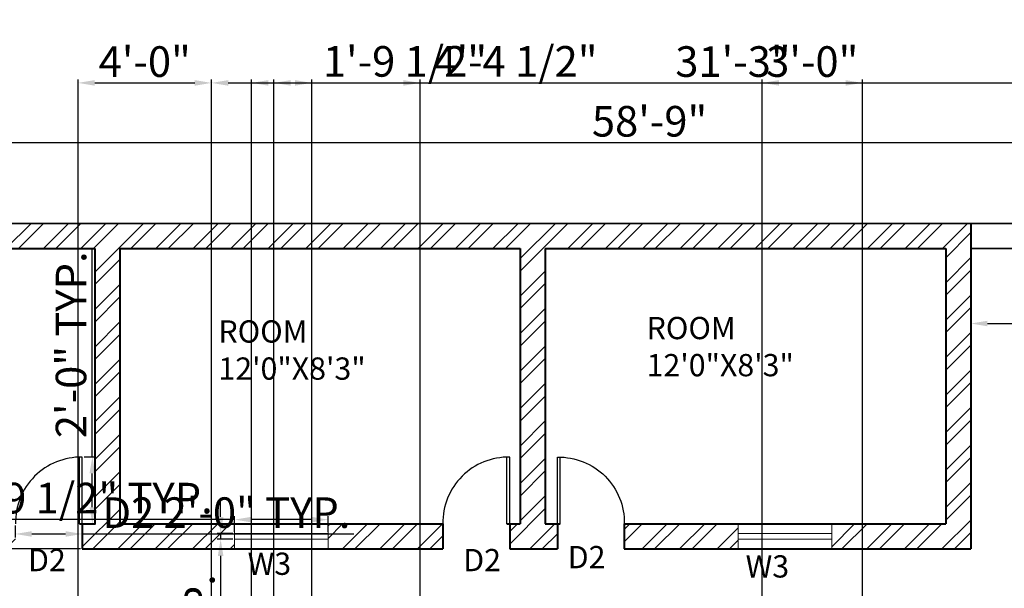
# Model space of a CAD drawing. Units: inches. Extents: x 2069 to 3028, y 691 to 1726.
# Tile 9 of 10: x 2268 to 2622, y 1521 to 1726. Entities that reach past the tile are written whole.
import ezdxf

# ---------------------------------------------------------------- set-up
doc = ezdxf.new("R2010")
doc.units = ezdxf.units.IN
for name, color, linetype, lineweight in [('A-ANNO-DIMS', 2, 'Continuous', 18), ('A-DOOR', 3, 'Continuous', 25), ('A-GLAZ', 4, 'Continuous', 20), ('A-WALL', 7, 'Continuous', 40), ('L-SITE-WALL', 7, 'Continuous', 35)]:
    doc.layers.add(name, color=color, linetype=linetype, lineweight=lineweight)
for name, color, linetype, lineweight, true_color in [('A-ANNO-TEXT', 11, 'Continuous', 18, 0xf27172), ('A-AREA-IDEN', 11, 'Continuous', 25, 0xf27172), ('A-WALL-PATT', 143, 'Continuous', 13, 0x7aafdf)]:
    doc.layers.add(name, color=color, linetype=linetype, lineweight=lineweight, true_color=true_color)
doc.styles.get("Standard").update_dxf_attribs({"font": 'arial.ttf'})
doc.dimstyles.new('ISO-25', dxfattribs={"dimtxt": 11, "dimasz": 6, "dimexe": 1.25, "dimexo": 0.625, "dimtad": 1, "dimlunit": 3, "dimtxsty": 'Standard', "dimcen": 2.5, "dimclrd": 3, "dimclre": 5, "dimclrt": 6, "dimadec": 0, "dimazin": 0, "dimtfac": 1, "dimtmove": 0, "dimatfit": 3, "dimfxl": 1, "dimarcsym": 0})

# ---------------------------------------------------------------- blocks, each defined once
blk = doc.blocks.new('*D20')
at = {"layer": 'A-ANNO-DIMS', "color": 0, "lineweight": -2, "transparency": 16777216}
for p, q in [((2141.95, 1653.01), (2141.95, 1682.68)), ((2846.95, 1653.01), (2846.95, 1682.68)), ((2147.95, 1681.43), (2840.95, 1681.43))]:
    blk.add_line(p, q, dxfattribs=at)
at = {"layer": 'A-ANNO-DIMS', "color": 0, "transparency": 16777216}
for points in [[(2147.95, 1682.43), (2147.95, 1680.43), (2141.95, 1681.43)], [(2840.95, 1682.43), (2840.95, 1680.43), (2846.95, 1681.43)]]:
    blk.add_solid(points, dxfattribs=at)
at = {"layer": 'Defpoints', "color": 0, "transparency": 16777216}
for p in [(2846.95, 1681.43), (2141.95, 1652.39), (2846.95, 1652.39)]:
    blk.add_point(p, dxfattribs=at)
at = {"layer": 'A-ANNO-DIMS', "color": 0, "transparency": 16777216, "insert": (2494.45, 1687.67), "char_height": 11, "attachment_point": 5}
blk.add_mtext('58\'-9"', dxfattribs=at)
blk = doc.blocks.new('*D22')
at = {"layer": 'A-ANNO-DIMS', "color": 0, "lineweight": -2, "transparency": 16777216}
for p, q in [((2609.95, 1642.76), (2609.95, 1615.16)), ((2837.95, 1642.76), (2837.95, 1615.16)), ((2615.95, 1616.41), (2831.95, 1616.41))]:
    blk.add_line(p, q, dxfattribs=at)
at = {"layer": 'A-ANNO-DIMS', "color": 0, "transparency": 16777216}
for points in [[(2615.95, 1617.41), (2615.95, 1615.41), (2609.95, 1616.41)], [(2831.95, 1617.41), (2831.95, 1615.41), (2837.95, 1616.41)]]:
    blk.add_solid(points, dxfattribs=at)
at = {"layer": 'Defpoints', "color": 0, "transparency": 16777216}
for p in [(2609.95, 1643.39), (2837.95, 1643.39), (2837.95, 1616.41)]:
    blk.add_point(p, dxfattribs=at)
at = {"layer": 'A-ANNO-DIMS', "color": 0, "transparency": 16777216, "insert": (2723.95, 1622.65), "char_height": 11, "attachment_point": 5}
blk.add_mtext("19'", dxfattribs=at)
blk = doc.blocks.new('DOOR-SWING-24IN')
for p, q in [((-1, 0), (-1, 24)), ((0, 0), (0, 24))]:
    blk.add_line(p, q)
blk.add_arc((-0.5, 0.5), 23.51, 88.7811, 181.2189)
blk = doc.blocks.new('WINDOW-SASH-33_6IN')
for p, q in [((0, 0), (33.6, 0)), ((0, -2), (33.6, -2))]:
    blk.add_line(p, q)
blk = doc.blocks.new('*D60')
at = {"layer": 'A-ANNO-DIMS', "color": 3, "lineweight": -2, "transparency": 16777216}
for p, q in [((2345.25, 1545.93), (2217.55, 1545.93)), ((2372.85, 1545.93), (2351.25, 1545.93))]:
    blk.add_line(p, q, dxfattribs=at)
at = {"layer": 'A-ANNO-DIMS', "color": 5, "lineweight": -2, "transparency": 16777216}
for p, q in [((2345.25, 1541.51), (2345.25, 1547.18)), ((2378.85, 1541.51), (2378.85, 1547.18))]:
    blk.add_line(p, q, dxfattribs=at)
at = {"layer": 'A-ANNO-DIMS', "color": 3, "transparency": 16777216}
for points in [[(2351.25, 1546.93), (2351.25, 1544.93), (2345.25, 1545.93)], [(2372.85, 1546.93), (2372.85, 1544.93), (2378.85, 1545.93)]]:
    blk.add_solid(points, dxfattribs=at)
at = {"layer": 'Defpoints', "color": 0, "transparency": 16777216}
for p in [(2345.25, 1545.93), (2345.25, 1540.89), (2378.85, 1540.89)]:
    blk.add_point(p, dxfattribs=at)
at = {"layer": 'A-ANNO-DIMS', "color": 6, "transparency": 16777216, "insert": (2278.4, 1552.24), "char_height": 11, "attachment_point": 5}
blk.add_mtext('W3 2\'-9 1/2" TYP.', dxfattribs=at)
blk = doc.blocks.new('*D61')
at = {"layer": 'A-ANNO-DIMS', "color": 3, "lineweight": -2, "transparency": 16777216}
for p, q in [((2340.21, 1546.89), (2340.21, 1552.89)), ((2340.21, 1540.89), (2340.21, 1538.89)), ((2340.21, 1532.89), (2340.21, 1458.59))]:
    blk.add_line(p, q, dxfattribs=at)
at = {"layer": 'A-ANNO-DIMS', "color": 5, "lineweight": -2, "transparency": 16777216}
for p, q in [((2344.62, 1540.89), (2338.96, 1540.89)), ((2344.62, 1538.89), (2338.96, 1538.89))]:
    blk.add_line(p, q, dxfattribs=at)
at = {"layer": 'A-ANNO-DIMS', "color": 3, "transparency": 16777216}
for points in [[(2339.21, 1546.89), (2341.21, 1546.89), (2340.21, 1540.89)], [(2339.21, 1532.89), (2341.21, 1532.89), (2340.21, 1538.89)]]:
    blk.add_solid(points, dxfattribs=at)
at = {"layer": 'Defpoints', "color": 0, "transparency": 16777216}
for p in [(2345.25, 1540.89), (2340.21, 1538.89), (2345.25, 1538.89)]:
    blk.add_point(p, dxfattribs=at)
at = {"layer": 'A-ANNO-DIMS', "color": 6, "transparency": 16777216, "insert": (2333.97, 1492.74), "char_height": 11, "attachment_point": 5, "rotation": 90}
blk.add_mtext('0\'-2" TYP.', dxfattribs=at)
blk = doc.blocks.new('*D62')
at = {"layer": 'A-ANNO-DIMS', "color": 5, "lineweight": -2, "transparency": 16777216}
for p, q in [((2266.31, 1543.76), (2266.31, 1539.52)), ((2290.45, 1543.76), (2290.45, 1539.52))]:
    blk.add_line(p, q, dxfattribs=at)
at = {"layer": 'A-ANNO-DIMS', "color": 3, "lineweight": -2, "transparency": 16777216}
for p, q in [((2272.31, 1540.77), (2284.45, 1540.77)), ((2290.45, 1540.77), (2388.12, 1540.77))]:
    blk.add_line(p, q, dxfattribs=at)
at = {"layer": 'A-ANNO-DIMS', "color": 3, "transparency": 16777216}
for points in [[(2272.31, 1541.77), (2272.31, 1539.77), (2266.31, 1540.77)], [(2284.45, 1541.77), (2284.45, 1539.77), (2290.45, 1540.77)]]:
    blk.add_solid(points, dxfattribs=at)
at = {"layer": 'Defpoints', "color": 0, "transparency": 16777216}
for p in [(2266.31, 1544.39), (2290.45, 1544.39), (2290.45, 1540.77)]:
    blk.add_point(p, dxfattribs=at)
at = {"layer": 'A-ANNO-DIMS', "color": 6, "transparency": 16777216, "insert": (2342.28, 1547.01), "char_height": 11, "attachment_point": 5}
blk.add_mtext('D2 2\'-0" TYP.', dxfattribs=at)
blk = doc.blocks.new('*D63')
at = {"layer": 'A-ANNO-DIMS', "color": 3, "lineweight": -2, "transparency": 16777216}
for p, q in [((2294.07, 1568.52), (2294.07, 1643.01)), ((2294.07, 1550.39), (2294.07, 1562.52))]:
    blk.add_line(p, q, dxfattribs=at)
at = {"layer": 'A-ANNO-DIMS', "color": 5, "lineweight": -2, "transparency": 16777216}
for p, q in [((2291.08, 1568.52), (2295.32, 1568.52)), ((2291.08, 1544.39), (2295.32, 1544.39))]:
    blk.add_line(p, q, dxfattribs=at)
at = {"layer": 'A-ANNO-DIMS', "color": 3, "transparency": 16777216}
for points in [[(2293.07, 1562.52), (2295.07, 1562.52), (2294.07, 1568.52)], [(2293.07, 1550.39), (2295.07, 1550.39), (2294.07, 1544.39)]]:
    blk.add_solid(points, dxfattribs=at)
at = {"layer": 'Defpoints', "color": 0, "transparency": 16777216}
for p in [(2290.45, 1568.52), (2294.07, 1568.52), (2290.45, 1544.39)]:
    blk.add_point(p, dxfattribs=at)
at = {"layer": 'A-ANNO-DIMS', "color": 6, "transparency": 16777216, "insert": (2287.83, 1608.77), "char_height": 11, "attachment_point": 5, "rotation": 90}
blk.add_mtext('2\'-0" TYP.', dxfattribs=at)
blk = doc.blocks.new('*D88')
at = {"layer": 'A-ANNO-DIMS', "color": 5, "lineweight": -2, "transparency": 16777216}
for p, q in [((2288.92, 738.01), (2288.92, 1704.14)), ((2336.92, 738.01), (2336.92, 1704.14))]:
    blk.add_line(p, q, dxfattribs=at)
at = {"layer": 'A-ANNO-DIMS', "color": 3, "lineweight": -2, "transparency": 16777216}
blk.add_line((2294.92, 1702.89), (2330.92, 1702.89), dxfattribs=at)
at = {"layer": 'A-ANNO-DIMS', "color": 3, "transparency": 16777216}
for points in [[(2294.92, 1703.89), (2294.92, 1701.89), (2288.92, 1702.89)], [(2330.92, 1703.89), (2330.92, 1701.89), (2336.92, 1702.89)]]:
    blk.add_solid(points, dxfattribs=at)
at = {"layer": 'Defpoints', "color": 0, "transparency": 16777216}
for p in [(2336.92, 1702.89), (2288.92, 737.39), (2336.92, 737.39)]:
    blk.add_point(p, dxfattribs=at)
at = {"layer": 'A-ANNO-DIMS', "color": 6, "transparency": 16777216, "insert": (2312.92, 1709.13), "char_height": 11, "attachment_point": 5}
blk.add_mtext('4\'-0"', dxfattribs=at)
blk = doc.blocks.new('*D89')
at = {"layer": 'A-ANNO-DIMS', "color": 5, "lineweight": -2, "transparency": 16777216}
for p, q in [((2336.92, 747.01), (2336.92, 1704.14)), ((2711.95, 747.01), (2711.95, 1704.14))]:
    blk.add_line(p, q, dxfattribs=at)
at = {"layer": 'A-ANNO-DIMS', "color": 3, "lineweight": -2, "transparency": 16777216}
blk.add_line((2342.92, 1702.89), (2705.95, 1702.89), dxfattribs=at)
at = {"layer": 'A-ANNO-DIMS', "color": 3, "transparency": 16777216}
for points in [[(2342.92, 1703.89), (2342.92, 1701.89), (2336.92, 1702.89)], [(2705.95, 1703.89), (2705.95, 1701.89), (2711.95, 1702.89)]]:
    blk.add_solid(points, dxfattribs=at)
at = {"layer": 'Defpoints', "color": 0, "transparency": 16777216}
for p in [(2711.95, 1702.89), (2336.92, 746.39), (2711.95, 746.39)]:
    blk.add_point(p, dxfattribs=at)
at = {"layer": 'A-ANNO-DIMS', "color": 6, "transparency": 16777216, "insert": (2524.44, 1709.13), "char_height": 11, "attachment_point": 5}
blk.add_mtext('31\'-3"', dxfattribs=at)
blk = doc.blocks.new('*D91')
at = {"layer": 'A-ANNO-DIMS', "color": 5, "lineweight": -2, "transparency": 16777216}
for p, q in [((2289.83, 1535.39), (2090.2, 1535.39)), ((2297.33, 1487.39), (2090.2, 1487.39))]:
    blk.add_line(p, q, dxfattribs=at)
at = {"layer": 'A-ANNO-DIMS', "color": 3, "lineweight": -2, "transparency": 16777216}
blk.add_line((2091.45, 1529.39), (2091.45, 1493.39), dxfattribs=at)
at = {"layer": 'A-ANNO-DIMS', "color": 3, "transparency": 16777216}
for points in [[(2090.45, 1529.39), (2092.45, 1529.39), (2091.45, 1535.39)], [(2090.45, 1493.39), (2092.45, 1493.39), (2091.45, 1487.39)]]:
    blk.add_solid(points, dxfattribs=at)
at = {"layer": 'Defpoints', "color": 0, "transparency": 16777216}
for p in [(2290.45, 1535.39), (2091.45, 1487.39), (2297.95, 1487.39)]:
    blk.add_point(p, dxfattribs=at)
at = {"layer": 'A-ANNO-DIMS', "color": 6, "transparency": 16777216, "insert": (2085.21, 1511.39), "char_height": 11, "attachment_point": 5, "rotation": 90}
blk.add_mtext('4\'-0"', dxfattribs=at)
blk = doc.blocks.new('*D92')
at = {"layer": 'A-ANNO-DIMS', "color": 5, "lineweight": -2, "transparency": 16777216}
for p, q in [((2359.37, 992.45), (2359.37, 1704.14)), ((2411.94, 992.45), (2411.94, 1704.14))]:
    blk.add_line(p, q, dxfattribs=at)
at = {"layer": 'A-ANNO-DIMS', "color": 3, "lineweight": -2, "transparency": 16777216}
for p, q in [((2365.37, 1702.89), (2405.94, 1702.89)), ((2411.94, 1702.89), (2474.5, 1702.89))]:
    blk.add_line(p, q, dxfattribs=at)
at = {"layer": 'A-ANNO-DIMS', "color": 3, "transparency": 16777216}
for points in [[(2365.37, 1703.89), (2365.37, 1701.89), (2359.37, 1702.89)], [(2405.94, 1703.89), (2405.94, 1701.89), (2411.94, 1702.89)]]:
    blk.add_solid(points, dxfattribs=at)
at = {"layer": 'Defpoints', "color": 0, "transparency": 16777216}
for p in [(2411.94, 1702.89), (2359.37, 991.83), (2411.94, 991.83)]:
    blk.add_point(p, dxfattribs=at)
at = {"layer": 'A-ANNO-DIMS', "color": 6, "transparency": 16777216, "insert": (2446.22, 1709.2), "char_height": 11, "attachment_point": 5}
blk.add_mtext('4\'-4 1/2"', dxfattribs=at)
blk = doc.blocks.new('*D95')
at = {"layer": 'A-ANNO-DIMS', "color": 5, "lineweight": -2, "transparency": 16777216}
for p, q in [((2351.35, 1134.01), (2351.35, 1704.14)), ((2372.95, 1134.01), (2372.95, 1704.14))]:
    blk.add_line(p, q, dxfattribs=at)
at = {"layer": 'A-ANNO-DIMS', "color": 3, "lineweight": -2, "transparency": 16777216}
for p, q in [((2357.35, 1702.89), (2366.95, 1702.89)), ((2372.95, 1702.89), (2434.04, 1702.89))]:
    blk.add_line(p, q, dxfattribs=at)
at = {"layer": 'A-ANNO-DIMS', "color": 3, "transparency": 16777216}
for points in [[(2357.35, 1703.89), (2357.35, 1701.89), (2351.35, 1702.89)], [(2366.95, 1703.89), (2366.95, 1701.89), (2372.95, 1702.89)]]:
    blk.add_solid(points, dxfattribs=at)
at = {"layer": 'Defpoints', "color": 0, "transparency": 16777216}
for p in [(2372.95, 1702.89), (2351.35, 1133.39), (2372.95, 1133.39)]:
    blk.add_point(p, dxfattribs=at)
at = {"layer": 'A-ANNO-DIMS', "color": 6, "transparency": 16777216, "insert": (2406.49, 1709.2), "char_height": 11, "attachment_point": 5}
blk.add_mtext('1\'-9 1/2"', dxfattribs=at)
blk = doc.blocks.new('*D96')
at = {"layer": 'A-ANNO-DIMS', "color": 5, "lineweight": -2, "transparency": 16777216}
for p, q in [((2534.95, 1066.51), (2534.95, 1704.14)), ((2570.95, 1066.51), (2570.95, 1704.14))]:
    blk.add_line(p, q, dxfattribs=at)
at = {"layer": 'A-ANNO-DIMS', "color": 3, "lineweight": -2, "transparency": 16777216}
blk.add_line((2540.95, 1702.89), (2564.95, 1702.89), dxfattribs=at)
at = {"layer": 'A-ANNO-DIMS', "color": 3, "transparency": 16777216}
for points in [[(2540.95, 1703.89), (2540.95, 1701.89), (2534.95, 1702.89)], [(2564.95, 1703.89), (2564.95, 1701.89), (2570.95, 1702.89)]]:
    blk.add_solid(points, dxfattribs=at)
at = {"layer": 'Defpoints', "color": 0, "transparency": 16777216}
for p in [(2570.95, 1702.89), (2534.95, 1065.89), (2570.95, 1065.89)]:
    blk.add_point(p, dxfattribs=at)
at = {"layer": 'A-ANNO-DIMS', "color": 6, "transparency": 16777216, "insert": (2552.95, 1709.13), "char_height": 11, "attachment_point": 5}
blk.add_mtext('3\'-0"', dxfattribs=at)

msp = doc.modelspace()

# ---------------------------------------------------------------- hatches: boundary and pattern name
at = {"layer": 'A-WALL-PATT'}
h = msp.add_hatch(dxfattribs=at)
h.set_pattern_fill('ANSI32', color=256)
h.paths.add_polyline_path([(2609.951, 1652.387), (2141.951, 1652.387), (2141.951, 1535.387), (2191.901, 1535.387), (2191.901, 1544.387), (2150.951, 1544.387), (2150.951, 1643.387), (2294.951, 1643.387), (2294.951, 1544.387), (2290.451, 1544.387), (2290.451, 1535.387), (2345.247, 1535.387), (2345.247, 1544.387), (2303.951, 1544.387), (2303.951, 1643.387), (2447.951, 1643.387), (2447.951, 1544.387), (2444.144, 1544.387), (2444.144, 1535.387), (2461.327, 1535.387), (2461.327, 1544.387), (2456.951, 1544.387), (2456.951, 1643.387), (2600.951, 1643.387), (2600.951, 1544.387), (2559.939, 1544.387), (2559.939, 1535.387), (2609.951, 1535.387)])
h.paths.add_polyline_path([(2266.451, 1544.387), (2225.501, 1544.387), (2225.501, 1535.387), (2266.451, 1535.387)], flags=17)
h.paths.add_polyline_path([(2420.144, 1544.387), (2378.847, 1544.387), (2378.847, 1535.387), (2420.144, 1535.387)], flags=17)
h.paths.add_polyline_path([(2526.339, 1544.387), (2485.327, 1544.387), (2485.327, 1535.387), (2526.339, 1535.387)], flags=17)

# ---------------------------------------------------------------- linework, layer by layer
at = {"layer": 'A-GLAZ'}
for p, q in [((2345.247, 1544.387), (2345.247, 1535.387)), ((2378.847, 1544.387), (2378.847, 1535.387)), ((2526.339, 1544.387), (2526.339, 1535.387)), ((2559.939, 1544.387), (2559.939, 1535.387))]:
    msp.add_line(p, q, dxfattribs=at)
at = {"layer": 'A-WALL'}
for p, q in [((2609.951, 1652.387), (2609.951, 1535.387)), ((2150.951, 1643.387), (2294.951, 1643.387)), ((2294.951, 1643.387), (2294.951, 1544.387)), ((2303.951, 1643.387), (2303.951, 1544.387)), ((2303.951, 1643.387), (2447.951, 1643.387)), ((2447.951, 1643.387), (2447.951, 1544.387)), ((2456.951, 1643.387), (2456.951, 1544.387)), ((2456.951, 1643.387), (2600.951, 1643.387)), ((2600.951, 1643.387), (2600.951, 1544.387)), ((2289.451, 1544.387), (2294.951, 1544.387)), ((2290.451, 1544.387), (2290.451, 1535.387)), ((2303.951, 1544.387), (2420.144, 1544.387)), ((2420.144, 1544.387), (2420.144, 1535.387)), ((2443.144, 1544.387), (2447.951, 1544.387)), ((2444.144, 1544.387), (2444.144, 1535.387)), ((2456.951, 1544.387), (2462.327, 1544.387)), ((2461.327, 1544.387), (2461.327, 1535.387)), ((2485.327, 1544.387), (2485.327, 1535.387)), ((2485.327, 1544.387), (2600.951, 1544.387)), ((2290.451, 1535.387), (2420.144, 1535.387)), ((2444.144, 1535.387), (2461.327, 1535.387)), ((2485.327, 1535.387), (2609.951, 1535.387))]:
    msp.add_line(p, q, dxfattribs=at)
at = {"layer": 'L-SITE-WALL'}
for p, q in [((2141.951, 1652.387), (2846.951, 1652.387)), ((2609.951, 1643.387), (2837.951, 1643.387))]:
    msp.add_line(p, q, dxfattribs=at)

# ---------------------------------------------------------------- block references
at = {"layer": 'A-DOOR'}
for p in [(2290.451, 1544.387), (2444.144, 1544.387)]:
    msp.add_blockref('DOOR-SWING-24IN', p, dxfattribs=at)
at = {"layer": 'A-DOOR', "extrusion": (0, 0, -1), "zscale": -1}
msp.add_blockref('DOOR-SWING-24IN', (-2461.327, 1544.387), dxfattribs=at)
at = {"layer": 'A-GLAZ', "rotation": 180}
for p in [(2378.847, 1538.887), (2559.939, 1538.887)]:
    msp.add_blockref('WINDOW-SASH-33_6IN', p, dxfattribs=at)

# ---------------------------------------------------------------- texts
at = {"layer": 'A-ANNO-TEXT', "char_height": 8, "attachment_point": 1}
for s, insert in [('{\\fArial|b1|i0|c0|p34;D2}', (2465.022, 1536.448)), ('{\\fArial|b1|i0|c0|p34;D2}', (2270.967, 1535.387)), ('{\\fArial|b1|i0|c0|p34;W3}', (2349.915, 1534.072)), ('{\\fArial|b1|i0|c0|p34;D2}', (2427.451, 1535.387)), ('{\\fArial|b1|i0|c0|p34;W3}', (2528.985, 1533.11))]:
    msp.add_mtext_dynamic_manual_height_columns(s, width=34.05605, gutter_width=12.5, heights=[0], dxfattribs=dict(at, insert=insert))
at = {"layer": 'A-AREA-IDEN', "char_height": 8, "attachment_point": 1}
for insert in [(2493.376, 1618.781), (2339.407, 1617.55)]:
    msp.add_mtext_dynamic_manual_height_columns('ROOM\\P12\'0"X8\'3"', width=119.20948, gutter_width=12.5, heights=[0], dxfattribs=dict(at, insert=insert))

# ---------------------------------------------------------------- dimensions: what is measured, and where the dimension line sits
at = {"layer": 'A-ANNO-DIMS'}
for base, p1, p2, override, picture, middle in [((2372.951, 1702.887), (2351.351, 1133.387), (2372.951, 1133.387), {"dimdec": 1, "dimlfac": 1, "dimrnd": 0, "dimzin": 1, "dimdsep": 46, "dimlunit": 4, "dimfrac": 2}, '*D95', (2406.495, 1709.199)), ((2411.936, 1702.887), (2359.366, 991.83), (2411.936, 991.83), {"dimdec": 1, "dimlfac": 1, "dimrnd": 0, "dimzin": 1, "dimdsep": 46, "dimlunit": 4, "dimfrac": 2}, '*D92', (2446.219, 1709.199)), ((2336.919, 1702.887), (2288.919, 737.387), (2336.919, 737.387), {"dimdec": 1, "dimlfac": 1, "dimrnd": 0, "dimzin": 1, "dimdsep": 46, "dimlunit": 4, "dimfrac": 2}, '*D88', (2312.919, 1709.128)), ((2711.951, 1702.887), (2336.919, 746.387), (2711.951, 746.387), {"dimdec": 1, "dimlfac": 1, "dimrnd": 0, "dimzin": 1, "dimdsep": 46, "dimlunit": 4, "dimfrac": 2}, '*D89', (2524.435, 1709.132)), ((2570.951, 1702.887), (2534.951, 1065.887), (2570.951, 1065.887), {"dimdec": 1, "dimlfac": 1, "dimrnd": 0, "dimzin": 1, "dimdsep": 46, "dimlunit": 4, "dimfrac": 2}, '*D96', (2552.951, 1709.132)), ((2846.951, 1681.427), (2141.951, 1652.387), (2846.951, 1652.387), {"dimclrd": 0, "dimclre": 0, "dimclrt": 0}, '*D20', (2494.451, 1687.669)), ((2837.951, 1616.413), (2609.951, 1643.387), (2837.951, 1643.387), {"dimclrd": 0, "dimclre": 0, "dimclrt": 0}, '*D22', (2723.951, 1622.654))]:
    dim = msp.add_linear_dim(base=base, p1=p1, p2=p2, dimstyle='ISO-25', override=override, dxfattribs=at)
    dim.commit()
    dim.dimension.update_dxf_attribs({"geometry": picture, "text_midpoint": middle})
for base, p1, p2, angle, text, picture, middle in [((2294.072, 1568.523), (2290.451, 1544.387), (2290.451, 1568.523), 90, '<> TYP.', '*D63', (2287.83, 1608.767)), ((2345.247, 1545.927), (2378.847, 1540.887), (2345.247, 1540.887), 180, 'W3 <> TYP.', '*D60', (2278.396, 1552.243)), ((2340.207, 1538.887), (2345.247, 1540.887), (2345.247, 1538.887), 270, '<> TYP.', '*D61', (2333.966, 1492.736))]:
    dim = msp.add_linear_dim(base=base, p1=p1, p2=p2, angle=angle, text=text, dimstyle='ISO-25', override={"dimdec": 1, "dimlfac": 1, "dimrnd": 0, "dimzin": 1, "dimdsep": 46, "dimlunit": 4, "dimfrac": 2}, dxfattribs=at)
    dim.commit()
    dim.dimension.update_dxf_attribs({"geometry": picture, "text_midpoint": middle})
dim = msp.add_linear_dim(base=(2290.451, 1540.766), p1=(2266.315, 1544.387), p2=(2290.451, 1544.387), text='D2 <> TYP.', dimstyle='ISO-25', override={"dimdec": 1, "dimlfac": 1, "dimrnd": 0, "dimzin": 1, "dimdsep": 46, "dimlunit": 4, "dimfrac": 2}, dxfattribs=at)
dim.commit()
dim.dimension.update_dxf_attribs({"geometry": '*D62', "text_midpoint": (2342.284, 1547.007)})
dim = msp.add_linear_dim(base=(2091.451, 1487.387), p1=(2290.451, 1535.387), p2=(2297.951, 1487.387), angle=90, dimstyle='ISO-25', override={"dimdec": 1, "dimlfac": 1, "dimrnd": 0, "dimzin": 1, "dimdsep": 46, "dimlunit": 4, "dimfrac": 2}, dxfattribs=at)
dim.commit()
dim.dimension.update_dxf_attribs({"geometry": '*D91', "text_midpoint": (2085.21, 1511.387)})

doc.saveas('drawing.dxf')
